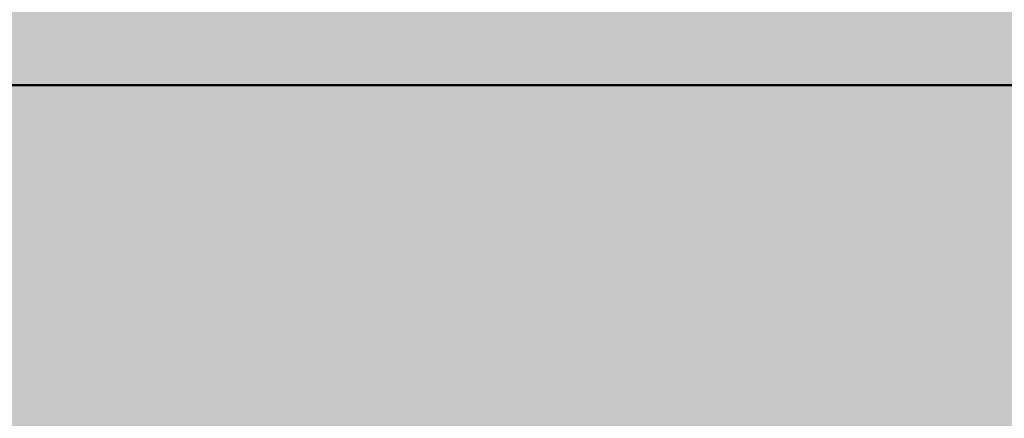
# Model space of a CAD drawing. Units: millimetres. Extents: x 0 to 2267, y 0 to 1823.
# Tile 129 of 256: x 1605.705 to 1611.042, y 1230.439 to 1232.602. Entities that reach past the tile are written whole.
import ezdxf

# ---------------------------------------------------------------- set-up
doc = ezdxf.new("R2010")
doc.units = ezdxf.units.MM
doc.header["$MEASUREMENT"] = 0
doc.layers.add('M-HATC', color=252, linetype='Continuous', lineweight=18)
doc.layers.add('M-OUTL', color=7, linetype='Continuous', lineweight=50)

msp = doc.modelspace()

# ---------------------------------------------------------------- hatches: boundary and pattern name
at = {"layer": 'M-HATC'}
h = msp.add_hatch(color=256, dxfattribs=at)
h.dxf.hatch_style = 1
h.paths.add_polyline_path([(2065.771, 1618.062, 0.236068), (2055.771, 1638.062), (1381.0868, 1638.062, 0.236068), (1371.0868, 1618.062), (1371.0868, 1603.062), (2055.771, 1603.062), (2065.771, 1603.062)])
h.paths.add_polyline_path([(2062.7718, 1550.2964), (2062.7718, 1560.2964), (1374.086, 1560.2964), (1374.086, 1550.2964), (1374.086, 1540.2964), (1384.086, 1540.2964), (1389.086, 1540.2964), (2062.7718, 1540.2964)])
h.paths.add_polyline_path([(1930.9289, 1282.7656), (1505.9289, 1282.7656), (1587.6276, 1235.5968, 0.131652), (1600.1276, 1232.2475), (1836.7302, 1232.2475, 0.131652), (1849.2302, 1235.5968)])
h.paths.add_polyline_path([(1930.9289, 1117.4171), (1905.9289, 1117.4171), (1505.9289, 1117.4171), (1505.9289, 1077.4171), (1930.9289, 1077.4171)])
h = msp.add_hatch(color=256, dxfattribs=at)
h.dxf.hatch_style = 1
h.paths.add_polyline_path([(2055.771, 1603.062), (1381.0868, 1603.062), (1381.0868, 1598.062), (2055.771, 1598.062)])
h.paths.add_polyline_path([(2055.771, 1598.062), (1381.0868, 1598.062), (1381.0868, 1593.062), (2055.771, 1593.062)])
h.paths.add_polyline_path([(2051.3074, 1536.7609), (1385.5504, 1536.7609), (1385.5504, 1526.7609), (1387.5504, 1526.7609), (1388.5366, 1525.0528), (1385.3319, 1521.2335), (1385.3319, 1521.2226), (2050.2542, 1522.7491), (2048.3212, 1525.0528), (2049.3074, 1526.7609), (2051.3074, 1526.7609)])
edge = h.paths.add_edge_path()
edge.add_arc((1847.5345, 1379.1492), 135, 222.603061, 222.890851, ccw=False)
edge.add_line((1748.1663, 1287.7656), (1683.0921, 1287.7656))
edge.add_arc((1583.7239, 1379.1492), 135, 317.109149, 317.396939, ccw=False)
edge.add_arc((1678.9686, 1290.6707), 5, 222.8909, 317.1091, ccw=False)
edge.add_arc((1774.2133, 1379.1492), 135, 222.603061, 222.890851, ccw=False)
edge.add_line((1674.8451, 1287.7656), (1609.7709, 1287.7656))
edge.add_arc((1510.4027, 1379.1492), 135, 317.109149, 317.396939, ccw=False)
edge.add_arc((1605.6474, 1290.6707), 5, 222.8909, 317.1091, ccw=False)
edge.add_arc((1700.8921, 1379.1492), 135, 222.603061, 222.890851, ccw=False)
edge.add_line((1601.5239, 1287.7656), (1536.4497, 1287.7656))
edge.add_arc((1437.0815, 1379.1492), 135, 317.109149, 317.396939, ccw=False)
edge.add_arc((1532.3262, 1290.6707), 5, 222.8909, 317.1091, ccw=False)
edge.add_arc((1627.5709, 1379.1492), 135, 222.603061, 222.890851, ccw=False)
edge.add_line((1528.2027, 1287.7656), (1505.9289, 1287.7656))
edge.add_spline(control_points=[(1505.9289, 1287.7656), (1504.2622, 1287.7656), (1504.2622, 1282.7656), (1505.9289, 1282.7656)], knot_values=[0, 0, 0, 0, 5, 5, 5, 5], degree=3, periodic=0)
edge.add_line((1505.9289, 1282.7656), (1930.9289, 1282.7656))
edge.add_spline(control_points=[(1930.9289, 1282.7656), (1932.5956, 1282.7656), (1932.5956, 1287.7656), (1930.9289, 1287.7656)], knot_values=[0, 0, 0, 0, 5, 5, 5, 5], degree=3, periodic=0)
edge.add_line((1930.9289, 1287.7656), (1903.0557, 1287.7656))
edge.add_arc((1803.6875, 1379.1492), 135, 317.109149, 317.396939, ccw=False)
edge.add_arc((1898.9322, 1290.6707), 5, 222.8909, 317.1091, ccw=False)
edge.add_arc((1994.1769, 1379.1492), 135, 222.603061, 222.890851, ccw=False)
edge.add_line((1894.8087, 1287.7656), (1829.7345, 1287.7656))
edge.add_arc((1730.3663, 1379.1492), 135, 317.109149, 317.396939, ccw=False)
edge.add_arc((1825.611, 1290.6707), 5, 222.8909, 317.1091, ccw=False)
edge.add_arc((1920.8557, 1379.1492), 135, 222.603061, 222.890851, ccw=False)
edge.add_line((1821.4875, 1287.7656), (1756.4133, 1287.7656))
edge.add_arc((1657.0451, 1379.1492), 135, 317.109149, 317.396939, ccw=False)
edge.add_arc((1752.2898, 1290.6707), 5, 222.8909, 317.1091, ccw=False)
edge = h.paths.add_edge_path()
edge.add_spline(control_points=[(1843.4289, 1227.2475), (1845.0956, 1227.2475), (1845.0956, 1232.2475), (1843.4289, 1232.2475)], knot_values=[0, 0, 0, 0, 5, 5, 5, 5], degree=3, periodic=0)
edge.add_line((1843.4289, 1232.2475), (1593.4289, 1232.2475))
edge.add_spline(control_points=[(1593.4289, 1232.2475), (1591.7622, 1232.2475), (1591.7622, 1227.2475), (1593.4289, 1227.2475)], knot_values=[0, 0, 0, 0, 5, 5, 5, 5], degree=3, periodic=0)
edge.add_line((1593.4289, 1227.2475), (1843.4289, 1227.2475))
h.paths.add_polyline_path([(1905.9289, 1127.4171), (1530.9289, 1127.4171, 0.414214), (1520.9289, 1117.4171), (1530.9289, 1117.4171), (1915.9289, 1117.4171, 0.414214)])
edge = h.paths.add_edge_path()
edge.add_arc((1397.0858, 1498.4078), 12.7299, 90.78215, 190.87871, ccw=False)
edge.add_line((1396.912, 1511.1365), (1428.0097, 1511.3488))
edge.add_line((1428.0097, 1511.3488), (1433.0097, 1511.3488))
edge.add_line((1433.0097, 1511.3488), (1434.439, 1511.3488))
edge.add_arc((1419.474, 1498.0804), 20, 41.561, 74.08211)
edge.add_line((1424.9592, 1517.3135), (1399.9351, 1517.2561))
edge.add_spline(control_points=[(1399.9307, 1517.2561), (1399.884, 1517.2131), (1399.8328, 1517.1689), (1399.7774, 1517.1236)], knot_values=[11.567499, 11.567499, 11.567499, 11.567499, 11.814249, 11.814249, 11.814249, 11.814249], degree=3, periodic=0)
edge.add_spline(control_points=[(1399.6328, 1517.0099), (1399.5831, 1516.9721), (1399.5307, 1516.9338), (1399.4759, 1516.8947)], knot_values=[11.167718, 11.167718, 11.167718, 11.167718, 11.365188, 11.365188, 11.365188, 11.365188], degree=3, periodic=0)
edge.add_spline(control_points=[(1399.3398, 1516.8001), (1399.1514, 1516.6719), (1398.9384, 1516.5377), (1398.704, 1516.3994)], knot_values=[10.376405, 10.376405, 10.376405, 10.376405, 11.00994, 11.00994, 11.00994, 11.00994], degree=3, periodic=0)
edge.add_spline(control_points=[(1398.6572, 1516.3719), (1398.5789, 1516.326), (1398.4983, 1516.2797), (1398.4155, 1516.2331)], knot_values=[10.125175, 10.125175, 10.125175, 10.125175, 10.334406, 10.334406, 10.334406, 10.334406], degree=3, periodic=0)
edge.add_spline(control_points=[(1398.2642, 1516.1487), (1398.196, 1516.1111), (1398.1263, 1516.0732), (1398.0555, 1516.0351)], knot_values=[9.832246, 9.832246, 9.832246, 9.832246, 9.999658, 9.999658, 9.999658, 9.999658], degree=3, periodic=0)
edge.add_spline(control_points=[(1397.9987, 1516.0048), (1397.7312, 1515.8621), (1397.446, 1515.7171), (1397.1466, 1515.5714)], knot_values=[9.161808, 9.161808, 9.161808, 9.161808, 9.787769, 9.787769, 9.787769, 9.787769], degree=3, periodic=0)
edge.add_spline(control_points=[(1397.1466, 1515.5714), (1396.8418, 1515.423), (1396.5222, 1515.274), (1396.1914, 1515.1262)], knot_values=[8.524455, 8.524455, 8.524455, 8.524455, 9.161808, 9.161808, 9.161808, 9.161808], degree=3, periodic=0)
edge.add_spline(control_points=[(1396.0777, 1515.0756), (1395.9854, 1515.0348), (1395.8922, 1514.994), (1395.7983, 1514.9534)], knot_values=[8.275193, 8.275193, 8.275193, 8.275193, 8.451726, 8.451726, 8.451726, 8.451726], degree=3, periodic=0)
edge.add_spline(control_points=[(1395.6018, 1514.8691), (1395.4997, 1514.8257), (1395.3968, 1514.7824), (1395.2932, 1514.7394)], knot_values=[7.962917, 7.962917, 7.962917, 7.962917, 8.152764, 8.152764, 8.152764, 8.152764], degree=3, periodic=0)
edge.add_spline(control_points=[(1395.2116, 1514.7057), (1394.8278, 1514.5475), (1394.4345, 1514.3929), (1394.0364, 1514.2442)], knot_values=[7.21254, 7.21254, 7.21254, 7.21254, 7.913148, 7.913148, 7.913148, 7.913148], degree=3, periodic=0)
edge.add_spline(control_points=[(1394.0364, 1514.2442), (1393.7076, 1514.1214), (1393.3754, 1514.0027), (1393.0427, 1513.8895)], knot_values=[6.633733, 6.633733, 6.633733, 6.633733, 7.21254, 7.21254, 7.21254, 7.21254], degree=3, periodic=0)
edge.add_spline(control_points=[(1392.8214, 1513.815), (1392.7198, 1513.7812), (1392.6181, 1513.7479), (1392.5166, 1513.7152)], knot_values=[6.328796, 6.328796, 6.328796, 6.328796, 6.505493, 6.505493, 6.505493, 6.505493], degree=3, periodic=0)
edge.add_spline(control_points=[(1392.5166, 1513.7152), (1392.3187, 1513.6515), (1392.1212, 1513.59), (1391.9244, 1513.531)], knot_values=[5.984605, 5.984605, 5.984605, 5.984605, 6.328796, 6.328796, 6.328796, 6.328796], degree=3, periodic=0)
edge.add_spline(control_points=[(1391.7915, 1513.4915), (1391.3122, 1513.3501), (1390.8384, 1513.2239), (1390.3784, 1513.1171)], knot_values=[5.066697, 5.066697, 5.066697, 5.066697, 5.907055, 5.907055, 5.907055, 5.907055], degree=3, periodic=0)
edge.add_spline(control_points=[(1390.3784, 1513.1171), (1390.1797, 1513.071), (1389.9836, 1513.0284), (1389.7907, 1512.9899)], knot_values=[4.70367, 4.70367, 4.70367, 4.70367, 5.066695, 5.066695, 5.066695, 5.066695], degree=3, periodic=0)
edge.add_spline(control_points=[(1389.422, 1512.9204), (1389.2459, 1512.8892), (1389.0729, 1512.8617), (1388.9036, 1512.8381)], knot_values=[4.130571, 4.130571, 4.130571, 4.130571, 4.469816, 4.469816, 4.469816, 4.469816], degree=3, periodic=0)
edge.add_spline(control_points=[(1388.9036, 1512.8381), (1388.591, 1512.7946), (1388.2911, 1512.7644), (1388.0071, 1512.7494)], knot_values=[3.504031, 3.504031, 3.504031, 3.504031, 4.130571, 4.130571, 4.130571, 4.130571], degree=3, periodic=0)
edge.add_spline(control_points=[(1387.9356, 1512.7459), (1387.8538, 1512.7423), (1387.7733, 1512.74), (1387.6944, 1512.739)], knot_values=[3.268866, 3.268866, 3.268866, 3.268866, 3.451164, 3.451164, 3.451164, 3.451164], degree=3, periodic=0)
edge.add_spline(control_points=[(1387.3351, 1512.7443), (1387.2076, 1512.7499), (1387.0847, 1512.7597), (1386.967, 1512.7739)], knot_values=[2.670686, 2.670686, 2.670686, 2.670686, 2.984, 2.984, 2.984, 2.984], degree=3, periodic=0)
edge.add_spline(control_points=[(1386.8327, 1512.7922), (1386.8209, 1512.7941), (1386.8092, 1512.7959), (1386.7975, 1512.7979)], knot_values=[2.516981, 2.516981, 2.516981, 2.516981, 2.549528, 2.549528, 2.549528, 2.549528], degree=3, periodic=0)
edge.add_spline(control_points=[(1386.4526, 1512.8735), (1386.4257, 1512.881), (1386.3993, 1512.889), (1386.3733, 1512.8972)], knot_values=[2.095869, 2.095869, 2.095869, 2.095869, 2.17941, 2.17941, 2.17941, 2.17941], degree=3, periodic=0)
edge.add_spline(control_points=[(1386.0691, 1513.0189), (1386.0634, 1513.0217), (1386.0577, 1513.0246), (1386.052, 1513.0275)], knot_values=[1.72453, 1.72453, 1.72453, 1.72453, 1.745933, 1.745933, 1.745933, 1.745933], degree=3, periodic=0)
edge.add_arc((1399.474, 1498.0804), 20, 131.82432, 180)
edge.add_arc((1630.3336, 1505.5484), 250.9708, 181.705176, 236.427975)
edge.add_arc((1605.3399, 1483.3044), 218.7822, 238.660829, 243.34961)
edge.add_arc((1647.0911, 1510.3592), 262.8986, 183.129836, 237.853442, ccw=False)
h.paths.add_polyline_path([(1406.5369, 1391.9644, 0.149382), (1491.5506, 1296.4418, -0.129517)], flags=17)
edge = h.paths.add_edge_path()
edge.add_arc((2037.3838, 1498.0804), 20, 0, 48.26587)
edge.add_spline(control_points=[(2050.6973, 1513.0052), (2050.6512, 1512.9847), (2050.6034, 1512.9655), (2050.5539, 1512.9477)], knot_values=[1.835652, 1.835652, 1.835652, 1.835652, 2.000781, 2.000781, 2.000781, 2.000781], degree=3, periodic=0)
edge.add_spline(control_points=[(2050.4616, 1512.9166), (2050.479, 1512.9221), (2050.4963, 1512.9277), (2050.5133, 1512.9335)], knot_values=[2.045477, 2.045477, 2.045477, 2.045477, 2.101389, 2.101389, 2.101389, 2.101389], degree=3, periodic=0)
edge.add_spline(control_points=[(2050.129, 1512.8342), (2050.1984, 1512.8473), (2050.2657, 1512.8623), (2050.3308, 1512.8792)], knot_values=[2.237629, 2.237629, 2.237629, 2.237629, 2.435841, 2.435841, 2.435841, 2.435841], degree=3, periodic=0)
edge.add_spline(control_points=[(2050.0946, 1512.8278), (2050.1061, 1512.8299), (2050.1176, 1512.832), (2050.129, 1512.8342)], knot_values=[2.435841, 2.435841, 2.435841, 2.435841, 2.468321, 2.468321, 2.468321, 2.468321], degree=3, periodic=0)
edge.add_spline(control_points=[(2049.7843, 1512.7851), (2049.8552, 1512.7922), (2049.9243, 1512.8008), (2049.9917, 1512.8109)], knot_values=[2.563852, 2.563852, 2.563852, 2.563852, 2.748541, 2.748541, 2.748541, 2.748541], degree=3, periodic=0)
edge.add_spline(control_points=[(2049.4052, 1512.7617), (2049.5364, 1512.7653), (2049.6629, 1512.773), (2049.7843, 1512.7851)], knot_values=[2.748541, 2.748541, 2.748541, 2.748541, 3.064882, 3.064882, 3.064882, 3.064882], degree=3, periodic=0)
edge.add_spline(control_points=[(2049.1698, 1512.7597), (2049.2336, 1512.7591), (2049.2965, 1512.7594), (2049.3584, 1512.7606)], knot_values=[3.102309, 3.102309, 3.102309, 3.102309, 3.2503, 3.2503, 3.2503, 3.2503], degree=3, periodic=0)
edge.add_spline(control_points=[(2048.8573, 1512.7691), (2048.9638, 1512.7638), (2049.068, 1512.7606), (2049.1698, 1512.7597)], knot_values=[3.2503, 3.2503, 3.2503, 3.2503, 3.486069, 3.486069, 3.486069, 3.486069], degree=3, periodic=0)
edge.add_spline(control_points=[(2048.6924, 1512.7789), (2048.3729, 1512.8009), (2048.0345, 1512.8411), (2047.6817, 1512.897)], knot_values=[3.606429, 3.606429, 3.606429, 3.606429, 4.2989, 4.2989, 4.2989, 4.2989], degree=3, periodic=0)
edge.add_spline(control_points=[(2047.6817, 1512.897), (2047.5458, 1512.9185), (2047.4077, 1512.9424), (2047.2678, 1512.9685)], knot_values=[4.2989, 4.2989, 4.2989, 4.2989, 4.565769, 4.565769, 4.565769, 4.565769], degree=3, periodic=0)
edge.add_spline(control_points=[(2047.2678, 1512.9685), (2047.1449, 1512.9914), (2047.0207, 1513.016), (2046.8951, 1513.0422)], knot_values=[4.565769, 4.565769, 4.565769, 4.565769, 4.799971, 4.799971, 4.799971, 4.799971], degree=3, periodic=0)
edge.add_spline(control_points=[(2046.8951, 1513.0422), (2046.5286, 1513.1188), (2046.1513, 1513.209), (2045.7676, 1513.3107)], knot_values=[4.799971, 4.799971, 4.799971, 4.799971, 5.483718, 5.483718, 5.483718, 5.483718], degree=3, periodic=0)
edge.add_spline(control_points=[(2045.7676, 1513.3107), (2045.3724, 1513.4154), (2044.9704, 1513.5322), (2044.5662, 1513.6588)], knot_values=[5.483718, 5.483718, 5.483718, 5.483718, 6.187866, 6.187866, 6.187866, 6.187866], degree=3, periodic=0)
edge.add_spline(control_points=[(2044.5662, 1513.6588), (2044.4149, 1513.7061), (2044.2633, 1513.7549), (2044.1116, 1513.8048)], knot_values=[6.187866, 6.187866, 6.187866, 6.187866, 6.451551, 6.451551, 6.451551, 6.451551], degree=3, periodic=0)
edge.add_spline(control_points=[(2044.1116, 1513.8048), (2043.9967, 1513.8427), (2043.8817, 1513.8813), (2043.7668, 1513.9205)], knot_values=[6.451551, 6.451551, 6.451551, 6.451551, 6.651434, 6.651434, 6.651434, 6.651434], degree=3, periodic=0)
edge.add_spline(control_points=[(2043.7668, 1513.9205), (2043.3716, 1514.0554), (2042.9774, 1514.1979), (2042.5886, 1514.3458)], knot_values=[6.651434, 6.651434, 6.651434, 6.651434, 7.338879, 7.338879, 7.338879, 7.338879], degree=3, periodic=0)
edge.add_spline(control_points=[(2042.5886, 1514.3458), (2042.1643, 1514.5071), (2041.7465, 1514.6749), (2041.3409, 1514.846)], knot_values=[7.338879, 7.338879, 7.338879, 7.338879, 8.089209, 8.089209, 8.089209, 8.089209], degree=3, periodic=0)
edge.add_spline(control_points=[(2041.3409, 1514.846), (2041.1028, 1514.9465), (2040.869, 1515.0481), (2040.6405, 1515.1502)], knot_values=[8.089209, 8.089209, 8.089209, 8.089209, 8.529587, 8.529587, 8.529587, 8.529587], degree=3, periodic=0)
edge.add_spline(control_points=[(2040.51, 1515.2089), (2040.0824, 1515.4022), (2039.6747, 1515.5971), (2039.295, 1515.7894)], knot_values=[8.613818, 8.613818, 8.613818, 8.613818, 9.44571, 9.44571, 9.44571, 9.44571], degree=3, periodic=0)
edge.add_spline(control_points=[(2039.295, 1515.7894), (2039.0618, 1515.9075), (2038.8391, 1516.0246), (2038.6288, 1516.1398)], knot_values=[9.44571, 9.44571, 9.44571, 9.44571, 9.956404, 9.956404, 9.956404, 9.956404], degree=3, periodic=0)
edge.add_spline(control_points=[(2038.6288, 1516.1398), (2038.5187, 1516.2001), (2038.4121, 1516.2598), (2038.309, 1516.3189)], knot_values=[9.956404, 9.956404, 9.956404, 9.956404, 10.223542, 10.223542, 10.223542, 10.223542], degree=3, periodic=0)
edge.add_spline(control_points=[(2038.309, 1516.3189), (2038.2138, 1516.3735), (2038.1216, 1516.4276), (2038.0328, 1516.481)], knot_values=[10.223542, 10.223542, 10.223542, 10.223542, 10.47051, 10.47051, 10.47051, 10.47051], degree=3, periodic=0)
edge.add_spline(control_points=[(2038.0328, 1516.481), (2037.7855, 1516.6296), (2037.5639, 1516.773), (2037.3722, 1516.909)], knot_values=[10.47051, 10.47051, 10.47051, 10.47051, 11.15767, 11.15767, 11.15767, 11.15767], degree=3, periodic=0)
edge.add_spline(control_points=[(2037.3722, 1516.909), (2037.2789, 1516.9752), (2037.1927, 1517.0396), (2037.1142, 1517.102)], knot_values=[11.15767, 11.15767, 11.15767, 11.15767, 11.49227, 11.49227, 11.49227, 11.49227], degree=3, periodic=0)
edge.add_spline(control_points=[(2036.8564, 1517.3259), (2036.9148, 1517.2692), (2036.9814, 1517.2103), (2037.0557, 1517.1492)], knot_values=[11.577341, 11.577341, 11.577341, 11.577341, 11.91035, 11.91035, 11.91035, 11.91035], degree=3, periodic=0)
edge.add_spline(control_points=[(2036.8074, 1517.3748), (2036.823, 1517.3587), (2036.8393, 1517.3424), (2036.8564, 1517.3259)], knot_values=[11.91035, 11.91035, 11.91035, 11.91035, 12.007402, 12.007402, 12.007402, 12.007402], degree=3, periodic=0)
edge.add_spline(control_points=[(2036.7017, 1517.494), (2036.7104, 1517.483), (2036.7196, 1517.4719), (2036.7291, 1517.4606)], knot_values=[12.184155, 12.184155, 12.184155, 12.184155, 12.255409, 12.255409, 12.255409, 12.255409], degree=3, periodic=0)
edge.add_spline(control_points=[(2036.6159, 1517.6205), (2036.62, 1517.613), (2036.6243, 1517.6055), (2036.6289, 1517.5979)], knot_values=[12.487913, 12.487913, 12.487913, 12.487913, 12.541035, 12.541035, 12.541035, 12.541035], degree=3, periodic=0)
edge.add_spline(control_points=[(2036.5635, 1517.786), (2036.5637, 1517.7794), (2036.5642, 1517.7726), (2036.565, 1517.7658)], knot_values=[12.911761, 12.911761, 12.911761, 12.911761, 12.968286, 12.968286, 12.968286, 12.968286], degree=3, periodic=0)
edge.add_spline(control_points=[(2036.6166, 1517.9304), (2036.6125, 1517.9259), (2036.6086, 1517.9212), (2036.6049, 1517.9165)], knot_values=[13.382527, 13.382527, 13.382527, 13.382527, 13.433791, 13.433791, 13.433791, 13.433791], degree=3, periodic=0)
edge.add_spline(control_points=[(2036.749, 1518.017), (2036.7361, 1518.0116), (2036.7239, 1518.006), (2036.7124, 1518.0002)], knot_values=[13.726299, 13.726299, 13.726299, 13.726299, 13.809928, 13.809928, 13.809928, 13.809928], degree=3, periodic=0)
edge.add_spline(control_points=[(2036.8604, 1518.0528), (2036.8386, 1518.0474), (2036.8181, 1518.0416), (2036.7988, 1518.0353)], knot_values=[13.910887, 13.910887, 13.910887, 13.910887, 14.02153, 14.02153, 14.02153, 14.02153], degree=3, periodic=0)
edge.add_line((2036.9639, 1518.0804), (2032.3838, 1518.0804))
edge.add_line((2032.3838, 1518.0804), (2027.3838, 1518.0804))
edge.add_line((2027.3838, 1518.0804), (2022.3838, 1518.0804))
edge.add_line((2022.3838, 1518.0804), (2017.3838, 1518.0804))
edge.add_arc((2017.3838, 1498.0804), 20, 90, 138.439)
edge.add_line((2002.4188, 1511.3488), (2003.8481, 1511.3488))
edge.add_line((2003.8481, 1511.3488), (2008.8481, 1511.3488))
edge.add_line((2008.8481, 1511.3488), (2039.772, 1511.1377))
edge.add_arc((2039.772, 1498.4078), 12.7299, -10.87871, 90, ccw=False)
edge.add_arc((1789.7668, 1510.3592), 262.8986, 302.146558, 356.870164, ccw=False)
edge.add_arc((1831.5179, 1483.3044), 218.7822, 296.65039, 301.339171)
edge.add_arc((1806.5242, 1505.5484), 250.9708, 303.572025, 358.294824)
h.paths.add_polyline_path([(2030.321, 1391.9644, -0.129517), (1945.3072, 1296.4418, 0.149382)], flags=17)
edge = h.paths.add_edge_path()
edge.add_spline(control_points=[(2037.2464, 1518.0821), (2037.2898, 1518.081), (2037.3355, 1518.0804), (2037.3838, 1518.0804)], knot_values=[0.000012, 0.000012, 0.000012, 0.000012, 0.144754, 0.144754, 0.144754, 0.144754], degree=3, periodic=0)
edge.add_line((2037.3357, 1518.0804), (2037.0096, 1518.0804))
edge.add_spline(control_points=[(2037.0096, 1518.0804), (2036.9822, 1518.0768), (2036.956, 1518.0727), (2036.9312, 1518.0681)], knot_values=[14.13465, 14.13465, 14.13465, 14.13465, 14.247197, 14.247197, 14.247197, 14.247197], degree=3, periodic=0)
edge.add_spline(control_points=[(2036.9312, 1518.0681), (2036.9276, 1518.0674), (2036.9241, 1518.0667), (2036.9205, 1518.0661)], knot_values=[14.118315, 14.118315, 14.118315, 14.118315, 14.13465, 14.13465, 14.13465, 14.13465], degree=3, periodic=0)
edge.add_spline(control_points=[(2036.9205, 1518.0661), (2036.9118, 1518.0644), (2036.9032, 1518.0626), (2036.8948, 1518.0608)], knot_values=[14.078086, 14.078086, 14.078086, 14.078086, 14.118315, 14.118315, 14.118315, 14.118315], degree=3, periodic=0)
edge.add_spline(control_points=[(2036.8948, 1518.0608), (2036.883, 1518.0583), (2036.8716, 1518.0556), (2036.8604, 1518.0528)], knot_values=[14.02153, 14.02153, 14.02153, 14.02153, 14.078086, 14.078086, 14.078086, 14.078086], degree=3, periodic=0)
edge.add_spline(control_points=[(2036.8604, 1518.0528), (2036.8386, 1518.0474), (2036.8181, 1518.0416), (2036.7988, 1518.0353)], knot_values=[13.910887, 13.910887, 13.910887, 13.910887, 14.02153, 14.02153, 14.02153, 14.02153], degree=3, periodic=0)
edge.add_spline(control_points=[(2036.7988, 1518.0353), (2036.7981, 1518.035), (2036.7974, 1518.0348), (2036.7967, 1518.0346)], knot_values=[13.906906, 13.906906, 13.906906, 13.906906, 13.910887, 13.910887, 13.910887, 13.910887], degree=3, periodic=0)
edge.add_spline(control_points=[(2036.7967, 1518.0346), (2036.7882, 1518.0318), (2036.7799, 1518.0289), (2036.7719, 1518.0259)], knot_values=[13.857826, 13.857826, 13.857826, 13.857826, 13.906906, 13.906906, 13.906906, 13.906906], degree=3, periodic=0)
edge.add_spline(control_points=[(2036.7719, 1518.0259), (2036.764, 1518.023), (2036.7564, 1518.02), (2036.749, 1518.017)], knot_values=[13.809928, 13.809928, 13.809928, 13.809928, 13.857826, 13.857826, 13.857826, 13.857826], degree=3, periodic=0)
edge.add_spline(control_points=[(2036.749, 1518.017), (2036.7361, 1518.0116), (2036.7239, 1518.006), (2036.7124, 1518.0002)], knot_values=[13.726299, 13.726299, 13.726299, 13.726299, 13.809928, 13.809928, 13.809928, 13.809928], degree=3, periodic=0)
edge.add_spline(control_points=[(2036.7124, 1518.0002), (2036.7121, 1518), (2036.7118, 1517.9999), (2036.7115, 1517.9997)], knot_values=[13.723993, 13.723993, 13.723993, 13.723993, 13.726299, 13.726299, 13.726299, 13.726299], degree=3, periodic=0)
edge.add_spline(control_points=[(2036.7115, 1517.9997), (2036.7063, 1517.9971), (2036.7013, 1517.9944), (2036.6965, 1517.9917)], knot_values=[13.686536, 13.686536, 13.686536, 13.686536, 13.723993, 13.723993, 13.723993, 13.723993], degree=3, periodic=0)
edge.add_spline(control_points=[(2036.6965, 1517.9917), (2036.6919, 1517.9891), (2036.6874, 1517.9865), (2036.6831, 1517.9839)], knot_values=[13.651251, 13.651251, 13.651251, 13.651251, 13.686536, 13.686536, 13.686536, 13.686536], degree=3, periodic=0)
edge.add_spline(control_points=[(2036.6831, 1517.9839), (2036.6764, 1517.9798), (2036.67, 1517.9757), (2036.6639, 1517.9714)], knot_values=[13.596804, 13.596804, 13.596804, 13.596804, 13.651251, 13.651251, 13.651251, 13.651251], degree=3, periodic=0)
edge.add_spline(control_points=[(2036.6639, 1517.9714), (2036.6636, 1517.9712), (2036.6633, 1517.9709), (2036.6629, 1517.9707)], knot_values=[13.593956, 13.593956, 13.593956, 13.593956, 13.596804, 13.596804, 13.596804, 13.596804], degree=3, periodic=0)
edge.add_spline(control_points=[(2036.6629, 1517.9707), (2036.6603, 1517.9689), (2036.6577, 1517.967), (2036.6552, 1517.9651)], knot_values=[13.570322, 13.570322, 13.570322, 13.570322, 13.593956, 13.593956, 13.593956, 13.593956], degree=3, periodic=0)
edge.add_spline(control_points=[(2036.6552, 1517.9651), (2036.6525, 1517.9631), (2036.6499, 1517.9611), (2036.6474, 1517.9591)], knot_values=[13.545477, 13.545477, 13.545477, 13.545477, 13.570322, 13.570322, 13.570322, 13.570322], degree=3, periodic=0)
edge.add_spline(control_points=[(2036.6474, 1517.9591), (2036.6472, 1517.9589), (2036.6471, 1517.9588), (2036.6469, 1517.9587)], knot_values=[13.543931, 13.543931, 13.543931, 13.543931, 13.545477, 13.545477, 13.545477, 13.545477], degree=3, periodic=0)
edge.add_spline(control_points=[(2036.6469, 1517.9587), (2036.6412, 1517.9541), (2036.6358, 1517.9494), (2036.6307, 1517.9447)], knot_values=[13.488237, 13.488237, 13.488237, 13.488237, 13.543931, 13.543931, 13.543931, 13.543931], degree=3, periodic=0)
edge.add_spline(control_points=[(2036.6307, 1517.9447), (2036.6282, 1517.9423), (2036.6257, 1517.9399), (2036.6233, 1517.9374)], knot_values=[13.460307, 13.460307, 13.460307, 13.460307, 13.488237, 13.488237, 13.488237, 13.488237], degree=3, periodic=0)
edge.add_spline(control_points=[(2036.6233, 1517.9374), (2036.6215, 1517.9356), (2036.6198, 1517.9338), (2036.6181, 1517.932)], knot_values=[13.439712, 13.439712, 13.439712, 13.439712, 13.460307, 13.460307, 13.460307, 13.460307], degree=3, periodic=0)
edge.add_spline(control_points=[(2036.6181, 1517.932), (2036.6176, 1517.9315), (2036.6171, 1517.9309), (2036.6166, 1517.9304)], knot_values=[13.433791, 13.433791, 13.433791, 13.433791, 13.439712, 13.439712, 13.439712, 13.439712], degree=3, periodic=0)
edge.add_spline(control_points=[(2036.6166, 1517.9304), (2036.6125, 1517.9259), (2036.6086, 1517.9212), (2036.6049, 1517.9165)], knot_values=[13.382527, 13.382527, 13.382527, 13.382527, 13.433791, 13.433791, 13.433791, 13.433791], degree=3, periodic=0)
edge.add_spline(control_points=[(2036.6049, 1517.9165), (2036.6026, 1517.9135), (2036.6004, 1517.9104), (2036.5982, 1517.9074)], knot_values=[13.350017, 13.350017, 13.350017, 13.350017, 13.382527, 13.382527, 13.382527, 13.382527], degree=3, periodic=0)
edge.add_spline(control_points=[(2036.5982, 1517.9074), (2036.5972, 1517.9059), (2036.5962, 1517.9043), (2036.5952, 1517.9028)], knot_values=[13.333922, 13.333922, 13.333922, 13.333922, 13.350017, 13.350017, 13.350017, 13.350017], degree=3, periodic=0)
edge.add_spline(control_points=[(2036.5952, 1517.9028), (2036.5945, 1517.9018), (2036.5939, 1517.9009), (2036.5933, 1517.8999)], knot_values=[13.323828, 13.323828, 13.323828, 13.323828, 13.333922, 13.333922, 13.333922, 13.333922], degree=3, periodic=0)
edge.add_spline(control_points=[(2036.5933, 1517.8999), (2036.5905, 1517.8955), (2036.5879, 1517.8909), (2036.5855, 1517.8864)], knot_values=[13.277545, 13.277545, 13.277545, 13.277545, 13.323828, 13.323828, 13.323828, 13.323828], degree=3, periodic=0)
edge.add_spline(control_points=[(2036.5855, 1517.8864), (2036.5836, 1517.8827), (2036.5817, 1517.8789), (2036.5801, 1517.8751)], knot_values=[13.240119, 13.240119, 13.240119, 13.240119, 13.277545, 13.277545, 13.277545, 13.277545], degree=3, periodic=0)
edge.add_spline(control_points=[(2036.5801, 1517.8751), (2036.5795, 1517.8739), (2036.579, 1517.8727), (2036.5785, 1517.8715)], knot_values=[13.228211, 13.228211, 13.228211, 13.228211, 13.240119, 13.240119, 13.240119, 13.240119], degree=3, periodic=0)
edge.add_spline(control_points=[(2036.5785, 1517.8715), (2036.578, 1517.8702), (2036.5774, 1517.869), (2036.5769, 1517.8677)], knot_values=[13.215717, 13.215717, 13.215717, 13.215717, 13.228211, 13.228211, 13.228211, 13.228211], degree=3, periodic=0)
edge.add_spline(control_points=[(2036.5769, 1517.8677), (2036.5755, 1517.864), (2036.5741, 1517.8603), (2036.5729, 1517.8565)], knot_values=[13.179847, 13.179847, 13.179847, 13.179847, 13.215717, 13.215717, 13.215717, 13.215717], degree=3, periodic=0)
edge.add_spline(control_points=[(2036.5729, 1517.8565), (2036.5713, 1517.8515), (2036.5699, 1517.8464), (2036.5687, 1517.8413)], knot_values=[13.132017, 13.132017, 13.132017, 13.132017, 13.179847, 13.179847, 13.179847, 13.179847], degree=3, periodic=0)
edge.add_spline(control_points=[(2036.5687, 1517.8413), (2036.5684, 1517.8402), (2036.5682, 1517.8392), (2036.568, 1517.8382)], knot_values=[13.122482, 13.122482, 13.122482, 13.122482, 13.132017, 13.132017, 13.132017, 13.132017], degree=3, periodic=0)
edge.add_spline(control_points=[(2036.568, 1517.8382), (2036.5676, 1517.8363), (2036.5672, 1517.8345), (2036.5669, 1517.8327)], knot_values=[13.105592, 13.105592, 13.105592, 13.105592, 13.122482, 13.122482, 13.122482, 13.122482], degree=3, periodic=0)
edge.add_spline(control_points=[(2036.5669, 1517.8327), (2036.5662, 1517.8292), (2036.5657, 1517.8257), (2036.5652, 1517.8222)], knot_values=[13.074063, 13.074063, 13.074063, 13.074063, 13.105592, 13.105592, 13.105592, 13.105592], degree=3, periodic=0)
edge.add_spline(control_points=[(2036.5652, 1517.8222), (2036.5652, 1517.8222), (2036.5652, 1517.8222), (2036.5652, 1517.8222)], knot_values=[13.074043, 13.074043, 13.074043, 13.074043, 13.074063, 13.074063, 13.074063, 13.074063], degree=3, periodic=0)
edge.add_spline(control_points=[(2036.5652, 1517.8222), (2036.5644, 1517.8164), (2036.5639, 1517.8106), (2036.5636, 1517.8046)], knot_values=[13.021884, 13.021884, 13.021884, 13.021884, 13.074043, 13.074043, 13.074043, 13.074043], degree=3, periodic=0)
edge.add_spline(control_points=[(2036.5636, 1517.8046), (2036.5636, 1517.804), (2036.5636, 1517.8034), (2036.5635, 1517.8028)], knot_values=[13.01674, 13.01674, 13.01674, 13.01674, 13.021884, 13.021884, 13.021884, 13.021884], degree=3, periodic=0)
edge.add_spline(control_points=[(2036.5635, 1517.8028), (2036.5634, 1517.8005), (2036.5634, 1517.7982), (2036.5634, 1517.7958)], knot_values=[12.996438, 12.996438, 12.996438, 12.996438, 13.01674, 13.01674, 13.01674, 13.01674], degree=3, periodic=0)
edge.add_spline(control_points=[(2036.5634, 1517.7958), (2036.5633, 1517.7926), (2036.5634, 1517.7893), (2036.5635, 1517.786)], knot_values=[12.968286, 12.968286, 12.968286, 12.968286, 12.996438, 12.996438, 12.996438, 12.996438], degree=3, periodic=0)
edge.add_spline(control_points=[(2036.5635, 1517.786), (2036.5637, 1517.7794), (2036.5642, 1517.7726), (2036.565, 1517.7658)], knot_values=[12.911761, 12.911761, 12.911761, 12.911761, 12.968286, 12.968286, 12.968286, 12.968286], degree=3, periodic=0)
edge.add_spline(control_points=[(2036.565, 1517.7658), (2036.565, 1517.7657), (2036.565, 1517.7656), (2036.565, 1517.7656)], knot_values=[12.911017, 12.911017, 12.911017, 12.911017, 12.911761, 12.911761, 12.911761, 12.911761], degree=3, periodic=0)
edge.add_spline(control_points=[(2036.565, 1517.7656), (2036.5654, 1517.7625), (2036.5658, 1517.7593), (2036.5663, 1517.7562)], knot_values=[12.88528, 12.88528, 12.88528, 12.88528, 12.911017, 12.911017, 12.911017, 12.911017], degree=3, periodic=0)
edge.add_spline(control_points=[(2036.5663, 1517.7562), (2036.5667, 1517.7534), (2036.5672, 1517.7506), (2036.5677, 1517.7478)], knot_values=[12.862519, 12.862519, 12.862519, 12.862519, 12.88528, 12.88528, 12.88528, 12.88528], degree=3, periodic=0)
edge.add_spline(control_points=[(2036.5677, 1517.7478), (2036.5678, 1517.7474), (2036.5679, 1517.7469), (2036.568, 1517.7465)], knot_values=[12.858885, 12.858885, 12.858885, 12.858885, 12.862519, 12.862519, 12.862519, 12.862519], degree=3, periodic=0)
edge.add_spline(control_points=[(2036.568, 1517.7465), (2036.5692, 1517.7399), (2036.5707, 1517.7332), (2036.5724, 1517.7264)], knot_values=[12.8053, 12.8053, 12.8053, 12.8053, 12.858885, 12.858885, 12.858885, 12.858885], degree=3, periodic=0)
edge.add_spline(control_points=[(2036.5724, 1517.7264), (2036.5734, 1517.7226), (2036.5745, 1517.7187), (2036.5756, 1517.7149)], knot_values=[12.775176, 12.775176, 12.775176, 12.775176, 12.8053, 12.8053, 12.8053, 12.8053], degree=3, periodic=0)
edge.add_spline(control_points=[(2036.5756, 1517.7149), (2036.5763, 1517.7125), (2036.577, 1517.7102), (2036.5778, 1517.7078)], knot_values=[12.756759, 12.756759, 12.756759, 12.756759, 12.775176, 12.775176, 12.775176, 12.775176], degree=3, periodic=0)
edge.add_spline(control_points=[(2036.5778, 1517.7078), (2036.5781, 1517.7067), (2036.5784, 1517.7057), (2036.5787, 1517.7047)], knot_values=[12.748742, 12.748742, 12.748742, 12.748742, 12.756759, 12.756759, 12.756759, 12.756759], degree=3, periodic=0)
edge.add_spline(control_points=[(2036.5787, 1517.7047), (2036.5808, 1517.6983), (2036.5831, 1517.6919), (2036.5856, 1517.6854)], knot_values=[12.69959, 12.69959, 12.69959, 12.69959, 12.748742, 12.748742, 12.748742, 12.748742], degree=3, periodic=0)
edge.add_spline(control_points=[(2036.5856, 1517.6854), (2036.5876, 1517.68), (2036.5898, 1517.6746), (2036.5921, 1517.6692)], knot_values=[12.659038, 12.659038, 12.659038, 12.659038, 12.69959, 12.69959, 12.69959, 12.69959], degree=3, periodic=0)
edge.add_spline(control_points=[(2036.5921, 1517.6692), (2036.594, 1517.6648), (2036.5959, 1517.6605), (2036.5979, 1517.6561)], knot_values=[12.626806, 12.626806, 12.626806, 12.626806, 12.659038, 12.659038, 12.659038, 12.659038], degree=3, periodic=0)
edge.add_spline(control_points=[(2036.5979, 1517.6561), (2036.5984, 1517.6551), (2036.5989, 1517.6541), (2036.5993, 1517.6531)], knot_values=[12.619394, 12.619394, 12.619394, 12.619394, 12.626806, 12.626806, 12.626806, 12.626806], degree=3, periodic=0)
edge.add_spline(control_points=[(2036.5993, 1517.6531), (2036.6043, 1517.6424), (2036.6099, 1517.6315), (2036.6159, 1517.6205)], knot_values=[12.541039, 12.541039, 12.541039, 12.541039, 12.619394, 12.619394, 12.619394, 12.619394], degree=3, periodic=0)
edge.add_spline(control_points=[(2036.6159, 1517.6205), (2036.6159, 1517.6205), (2036.6159, 1517.6205), (2036.6159, 1517.6205)], knot_values=[12.541035, 12.541035, 12.541035, 12.541035, 12.541039, 12.541039, 12.541039, 12.541039], degree=3, periodic=0)
edge.add_spline(control_points=[(2036.6159, 1517.6205), (2036.62, 1517.613), (2036.6243, 1517.6055), (2036.6289, 1517.5979)], knot_values=[12.487913, 12.487913, 12.487913, 12.487913, 12.541035, 12.541035, 12.541035, 12.541035], degree=3, periodic=0)
edge.add_spline(control_points=[(2036.6289, 1517.5979), (2036.6326, 1517.5916), (2036.6365, 1517.5853), (2036.6406, 1517.5789)], knot_values=[12.443982, 12.443982, 12.443982, 12.443982, 12.487913, 12.487913, 12.487913, 12.487913], degree=3, periodic=0)
edge.add_spline(control_points=[(2036.6406, 1517.5789), (2036.6414, 1517.5776), (2036.6423, 1517.5763), (2036.6431, 1517.5749)], knot_values=[12.434996, 12.434996, 12.434996, 12.434996, 12.443982, 12.443982, 12.443982, 12.443982], degree=3, periodic=0)
edge.add_spline(control_points=[(2036.6431, 1517.5749), (2036.6531, 1517.5596), (2036.6639, 1517.5439), (2036.6756, 1517.528)], knot_values=[12.329647, 12.329647, 12.329647, 12.329647, 12.434996, 12.434996, 12.434996, 12.434996], degree=3, periodic=0)
edge.add_spline(control_points=[(2036.6756, 1517.528), (2036.6839, 1517.5168), (2036.6925, 1517.5055), (2036.7017, 1517.494)], knot_values=[12.255409, 12.255409, 12.255409, 12.255409, 12.329647, 12.329647, 12.329647, 12.329647], degree=3, periodic=0)
edge.add_spline(control_points=[(2036.7017, 1517.494), (2036.7104, 1517.483), (2036.7196, 1517.4719), (2036.7291, 1517.4606)], knot_values=[12.184155, 12.184155, 12.184155, 12.184155, 12.255409, 12.255409, 12.255409, 12.255409], degree=3, periodic=0)
edge.add_spline(control_points=[(2036.7291, 1517.4606), (2036.7436, 1517.4435), (2036.759, 1517.4262), (2036.7753, 1517.4085)], knot_values=[12.075961, 12.075961, 12.075961, 12.075961, 12.184155, 12.184155, 12.184155, 12.184155], degree=3, periodic=0)
edge.add_spline(control_points=[(2036.7753, 1517.4085), (2036.7763, 1517.4075), (2036.7773, 1517.4064), (2036.7783, 1517.4054)], knot_values=[12.069502, 12.069502, 12.069502, 12.069502, 12.075961, 12.075961, 12.075961, 12.075961], degree=3, periodic=0)
edge.add_spline(control_points=[(2036.7783, 1517.4054), (2036.7877, 1517.3953), (2036.7974, 1517.385), (2036.8074, 1517.3748)], knot_values=[12.007402, 12.007402, 12.007402, 12.007402, 12.069502, 12.069502, 12.069502, 12.069502], degree=3, periodic=0)
edge.add_spline(control_points=[(2036.8074, 1517.3748), (2036.823, 1517.3587), (2036.8393, 1517.3424), (2036.8564, 1517.3259)], knot_values=[11.91035, 11.91035, 11.91035, 11.91035, 12.007402, 12.007402, 12.007402, 12.007402], degree=3, periodic=0)
edge.add_spline(control_points=[(2036.8564, 1517.3259), (2036.9148, 1517.2692), (2036.9814, 1517.2103), (2037.0557, 1517.1492)], knot_values=[11.577341, 11.577341, 11.577341, 11.577341, 11.91035, 11.91035, 11.91035, 11.91035], degree=3, periodic=0)
edge.add_spline(control_points=[(2037.0557, 1517.1492), (2037.0747, 1517.1336), (2037.0942, 1517.1179), (2037.1142, 1517.102)], knot_values=[11.49227, 11.49227, 11.49227, 11.49227, 11.577341, 11.577341, 11.577341, 11.577341], degree=3, periodic=0)
edge.add_spline(control_points=[(2037.1142, 1517.102), (2037.1927, 1517.0396), (2037.2789, 1516.9752), (2037.3722, 1516.909)], knot_values=[11.15767, 11.15767, 11.15767, 11.15767, 11.49227, 11.49227, 11.49227, 11.49227], degree=3, periodic=0)
edge.add_spline(control_points=[(2037.3722, 1516.909), (2037.5639, 1516.773), (2037.7855, 1516.6296), (2038.0328, 1516.481)], knot_values=[10.47051, 10.47051, 10.47051, 10.47051, 11.15767, 11.15767, 11.15767, 11.15767], degree=3, periodic=0)
edge.add_spline(control_points=[(2038.0328, 1516.481), (2038.1216, 1516.4276), (2038.2138, 1516.3735), (2038.309, 1516.3189)], knot_values=[10.223542, 10.223542, 10.223542, 10.223542, 10.47051, 10.47051, 10.47051, 10.47051], degree=3, periodic=0)
edge.add_spline(control_points=[(2038.309, 1516.3189), (2038.4121, 1516.2598), (2038.5187, 1516.2001), (2038.6288, 1516.1398)], knot_values=[9.956404, 9.956404, 9.956404, 9.956404, 10.223542, 10.223542, 10.223542, 10.223542], degree=3, periodic=0)
edge.add_spline(control_points=[(2038.6288, 1516.1398), (2038.8391, 1516.0246), (2039.0618, 1515.9075), (2039.295, 1515.7894)], knot_values=[9.44571, 9.44571, 9.44571, 9.44571, 9.956404, 9.956404, 9.956404, 9.956404], degree=3, periodic=0)
edge.add_spline(control_points=[(2039.295, 1515.7894), (2039.6747, 1515.5971), (2040.0824, 1515.4022), (2040.51, 1515.2089)], knot_values=[8.613818, 8.613818, 8.613818, 8.613818, 9.44571, 9.44571, 9.44571, 9.44571], degree=3, periodic=0)
edge.add_spline(control_points=[(2040.51, 1515.2089), (2040.5533, 1515.1893), (2040.5968, 1515.1697), (2040.6405, 1515.1502)], knot_values=[8.529587, 8.529587, 8.529587, 8.529587, 8.613818, 8.613818, 8.613818, 8.613818], degree=3, periodic=0)
edge.add_spline(control_points=[(2040.6405, 1515.1502), (2040.869, 1515.0481), (2041.1028, 1514.9465), (2041.3409, 1514.846)], knot_values=[8.089209, 8.089209, 8.089209, 8.089209, 8.529587, 8.529587, 8.529587, 8.529587], degree=3, periodic=0)
edge.add_spline(control_points=[(2041.3409, 1514.846), (2041.7465, 1514.6749), (2042.1643, 1514.5071), (2042.5886, 1514.3458)], knot_values=[7.338879, 7.338879, 7.338879, 7.338879, 8.089209, 8.089209, 8.089209, 8.089209], degree=3, periodic=0)
edge.add_spline(control_points=[(2042.5886, 1514.3458), (2042.9774, 1514.1979), (2043.3716, 1514.0554), (2043.7668, 1513.9205)], knot_values=[6.651434, 6.651434, 6.651434, 6.651434, 7.338879, 7.338879, 7.338879, 7.338879], degree=3, periodic=0)
edge.add_spline(control_points=[(2043.7668, 1513.9205), (2043.8817, 1513.8813), (2043.9967, 1513.8427), (2044.1116, 1513.8048)], knot_values=[6.451551, 6.451551, 6.451551, 6.451551, 6.651434, 6.651434, 6.651434, 6.651434], degree=3, periodic=0)
edge.add_spline(control_points=[(2044.1116, 1513.8048), (2044.2633, 1513.7549), (2044.4149, 1513.7061), (2044.5662, 1513.6588)], knot_values=[6.187866, 6.187866, 6.187866, 6.187866, 6.451551, 6.451551, 6.451551, 6.451551], degree=3, periodic=0)
edge.add_spline(control_points=[(2044.5662, 1513.6588), (2044.9704, 1513.5322), (2045.3724, 1513.4154), (2045.7676, 1513.3107)], knot_values=[5.483718, 5.483718, 5.483718, 5.483718, 6.187866, 6.187866, 6.187866, 6.187866], degree=3, periodic=0)
edge.add_spline(control_points=[(2045.7676, 1513.3107), (2046.1513, 1513.209), (2046.5286, 1513.1188), (2046.8951, 1513.0422)], knot_values=[4.799971, 4.799971, 4.799971, 4.799971, 5.483718, 5.483718, 5.483718, 5.483718], degree=3, periodic=0)
edge.add_spline(control_points=[(2046.8951, 1513.0422), (2047.0207, 1513.016), (2047.1449, 1512.9914), (2047.2678, 1512.9685)], knot_values=[4.565769, 4.565769, 4.565769, 4.565769, 4.799971, 4.799971, 4.799971, 4.799971], degree=3, periodic=0)
edge.add_spline(control_points=[(2047.2678, 1512.9685), (2047.4077, 1512.9424), (2047.5458, 1512.9185), (2047.6817, 1512.897)], knot_values=[4.2989, 4.2989, 4.2989, 4.2989, 4.565769, 4.565769, 4.565769, 4.565769], degree=3, periodic=0)
edge.add_spline(control_points=[(2047.6817, 1512.897), (2048.0345, 1512.8411), (2048.3729, 1512.8009), (2048.6924, 1512.7789)], knot_values=[3.606429, 3.606429, 3.606429, 3.606429, 4.2989, 4.2989, 4.2989, 4.2989], degree=3, periodic=0)
edge.add_spline(control_points=[(2048.6924, 1512.7789), (2048.7479, 1512.7751), (2048.8029, 1512.7718), (2048.8573, 1512.7691)], knot_values=[3.486069, 3.486069, 3.486069, 3.486069, 3.606429, 3.606429, 3.606429, 3.606429], degree=3, periodic=0)
edge.add_spline(control_points=[(2048.8573, 1512.7691), (2048.9638, 1512.7638), (2049.068, 1512.7606), (2049.1698, 1512.7597)], knot_values=[3.2503, 3.2503, 3.2503, 3.2503, 3.486069, 3.486069, 3.486069, 3.486069], degree=3, periodic=0)
edge.add_spline(control_points=[(2049.1698, 1512.7597), (2049.2336, 1512.7591), (2049.2965, 1512.7594), (2049.3584, 1512.7606)], knot_values=[3.102309, 3.102309, 3.102309, 3.102309, 3.2503, 3.2503, 3.2503, 3.2503], degree=3, periodic=0)
edge.add_spline(control_points=[(2049.3584, 1512.7606), (2049.3741, 1512.7609), (2049.3897, 1512.7613), (2049.4052, 1512.7617)], knot_values=[3.064882, 3.064882, 3.064882, 3.064882, 3.102309, 3.102309, 3.102309, 3.102309], degree=3, periodic=0)
edge.add_spline(control_points=[(2049.4052, 1512.7617), (2049.5364, 1512.7653), (2049.6629, 1512.773), (2049.7843, 1512.7851)], knot_values=[2.748541, 2.748541, 2.748541, 2.748541, 3.064882, 3.064882, 3.064882, 3.064882], degree=3, periodic=0)
edge.add_spline(control_points=[(2049.7843, 1512.7851), (2049.8552, 1512.7922), (2049.9243, 1512.8008), (2049.9917, 1512.8109)], knot_values=[2.563852, 2.563852, 2.563852, 2.563852, 2.748541, 2.748541, 2.748541, 2.748541], degree=3, periodic=0)
edge.add_spline(control_points=[(2049.9917, 1512.8109), (2050.0265, 1512.8161), (2050.0608, 1512.8218), (2050.0946, 1512.8278)], knot_values=[2.468321, 2.468321, 2.468321, 2.468321, 2.563852, 2.563852, 2.563852, 2.563852], degree=3, periodic=0)
edge.add_spline(control_points=[(2050.0946, 1512.8278), (2050.1061, 1512.8299), (2050.1176, 1512.832), (2050.129, 1512.8342)], knot_values=[2.435841, 2.435841, 2.435841, 2.435841, 2.468321, 2.468321, 2.468321, 2.468321], degree=3, periodic=0)
edge.add_spline(control_points=[(2050.129, 1512.8342), (2050.1984, 1512.8473), (2050.2657, 1512.8623), (2050.3308, 1512.8792)], knot_values=[2.237629, 2.237629, 2.237629, 2.237629, 2.435841, 2.435841, 2.435841, 2.435841], degree=3, periodic=0)
edge.add_spline(control_points=[(2050.3308, 1512.8792), (2050.3754, 1512.8908), (2050.4191, 1512.9032), (2050.4616, 1512.9166)], knot_values=[2.101389, 2.101389, 2.101389, 2.101389, 2.237629, 2.237629, 2.237629, 2.237629], degree=3, periodic=0)
edge.add_spline(control_points=[(2050.4616, 1512.9166), (2050.479, 1512.9221), (2050.4963, 1512.9277), (2050.5133, 1512.9335)], knot_values=[2.045477, 2.045477, 2.045477, 2.045477, 2.101389, 2.101389, 2.101389, 2.101389], degree=3, periodic=0)
edge.add_spline(control_points=[(2050.5133, 1512.9335), (2050.527, 1512.9382), (2050.5405, 1512.9429), (2050.5539, 1512.9477)], knot_values=[2.000781, 2.000781, 2.000781, 2.000781, 2.045477, 2.045477, 2.045477, 2.045477], degree=3, periodic=0)
edge.add_spline(control_points=[(2050.5539, 1512.9477), (2050.6034, 1512.9655), (2050.6512, 1512.9847), (2050.6973, 1513.0052)], knot_values=[1.835652, 1.835652, 1.835652, 1.835652, 2.000781, 2.000781, 2.000781, 2.000781], degree=3, periodic=0)
edge.add_arc((2037.3838, 1498.0804), 20, 48.26587, 90.12993)
edge = h.paths.add_edge_path(flags=16)
edge.add_spline(control_points=[(1386.1389, 1512.9859), (1388.92, 1511.7395), (1398.0387, 1515.5187), (1399.9307, 1517.2561)], knot_values=[1.831046, 1.831046, 1.831046, 1.831046, 11.814249, 11.814249, 11.814249, 11.814249], degree=3, periodic=0)
edge.add_line((1399.9307, 1517.2561), (1393.7435, 1517.2419))
edge.add_arc((1399.474, 1498.0804), 20, 106.6501, 131.8173)

# ---------------------------------------------------------------- linework, layer by layer
at = {"layer": 'M-OUTL'}
msp.add_line((1593.4289, 1232.2475), (1843.4289, 1232.2475), dxfattribs=at)

doc.saveas('drawing.dxf')
